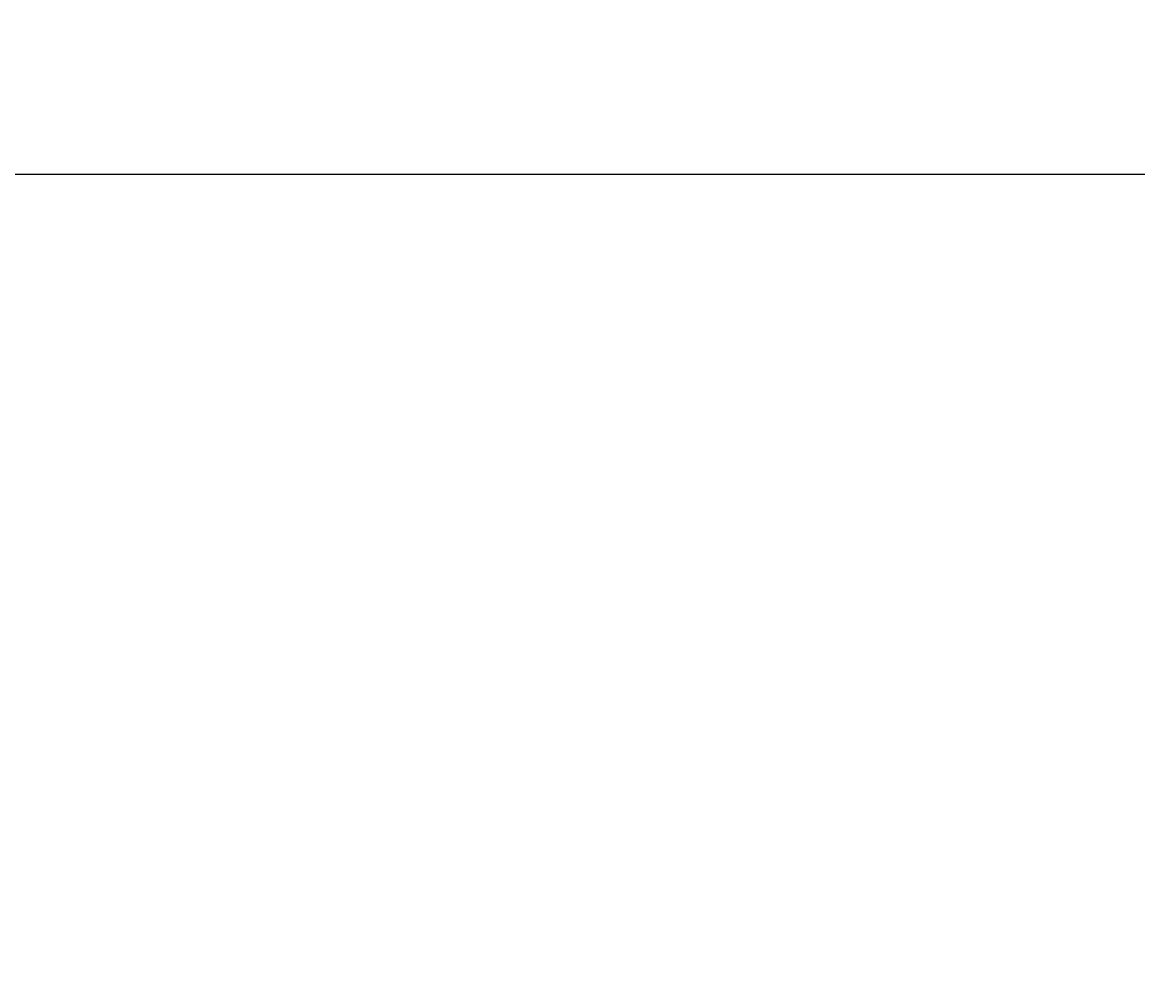
# Model space of a CAD drawing. Units: inches. Extents: x 35362 to 73946, y 43607 to 67532.
# Tile 106 of 134: x 50761 to 50905, y 48793 to 48917. Entities that reach past the tile are written whole.
import ezdxf

# ---------------------------------------------------------------- set-up
doc = ezdxf.new("R2010")
doc.units = ezdxf.units.IN
doc.header["$MEASUREMENT"] = 0
doc.layers.add('A-ANNO-DIMS', color=2, linetype='Continuous', lineweight=18)
doc.styles.get("Standard").update_dxf_attribs({"font": 'arial.ttf'})
doc.dimstyles.get("Standard").update_dxf_attribs({"dimtxt": 0.18, "dimasz": 0.18, "dimexe": 0.18, "dimexo": 0.0625, "dimgap": 0.09, "dimtad": 0, "dimtih": 1, "dimtoh": 1, "dimdec": 4, "dimzin": 0, "dimdsep": 46, "dimtxsty": 'Standard', "dimcen": 0.09, "dimadec": 0, "dimazin": 0, "dimtfac": 1, "dimtdec": 4, "dimtofl": 0, "dimtmove": 0, "dimatfit": 3, "dimfxl": 1, "dimtolj": 1, "dimtzin": 0, "dimarcsym": 0})

# ---------------------------------------------------------------- blocks, each defined once
blk = doc.blocks.new('*D11')
at = {"layer": 'A-ANNO-DIMS', "color": 0, "lineweight": -2, "transparency": 16777216}
for p, q in [((47978.66, 56028.77), (47978.66, 43606.68)), ((53109.76, 56028.77), (53109.76, 43606.68)), ((47978.84, 43606.86), (50543.87, 43606.86)), ((53109.58, 43606.86), (50544.55, 43606.86))]:
    blk.add_line(p, q, dxfattribs=at)
at = {"layer": 'A-ANNO-DIMS', "color": 0, "transparency": 16777216}
for points in [[(47978.84, 43606.89), (47978.84, 43606.83), (47978.66, 43606.86)], [(53109.58, 43606.89), (53109.58, 43606.83), (53109.76, 43606.86)]]:
    blk.add_solid(points, dxfattribs=at)
at = {"layer": 'Defpoints', "color": 0, "transparency": 16777216}
for p in [(47978.66, 56028.84), (53109.76, 56028.84), (53109.76, 43606.86)]:
    blk.add_point(p, dxfattribs=at)
at = {"layer": 'A-ANNO-DIMS', "color": 0, "transparency": 16777216, "insert": (50544.21, 43606.86), "char_height": 0.18, "attachment_point": 5}
blk.add_mtext('\\A1;5131', dxfattribs=at)
blk = doc.blocks.new('*D13')
at = {"layer": 'A-ANNO-DIMS', "color": 0, "lineweight": -2, "transparency": 16777216}
for p, q in [((48373.49, 51694.02), (48373.49, 43606.68)), ((51029.04, 51694.02), (51029.04, 43606.68)), ((48373.67, 43606.86), (49700.8, 43606.86)), ((51028.86, 43606.86), (49701.73, 43606.86))]:
    blk.add_line(p, q, dxfattribs=at)
at = {"layer": 'A-ANNO-DIMS', "color": 0, "transparency": 16777216}
for points in [[(48373.67, 43606.89), (48373.67, 43606.83), (48373.49, 43606.86)], [(51028.86, 43606.89), (51028.86, 43606.83), (51029.04, 43606.86)]]:
    blk.add_solid(points, dxfattribs=at)
at = {"layer": 'Defpoints', "color": 0, "transparency": 16777216}
for p in [(48373.49, 51694.09), (51029.04, 51694.09), (51029.04, 43606.86)]:
    blk.add_point(p, dxfattribs=at)
at = {"layer": 'A-ANNO-DIMS', "color": 0, "transparency": 16777216, "insert": (49701.27, 43606.86), "char_height": 0.18, "attachment_point": 5}
blk.add_mtext('\\A1;2655.6', dxfattribs=at)
blk = doc.blocks.new('*D17')
at = {"layer": 'A-ANNO-DIMS', "color": 0, "lineweight": -2, "transparency": 16777216}
for p, q in [((49923.31, 61293.22), (49923.31, 43606.68)), ((51913.93, 61293.22), (51913.93, 43606.68)), ((49923.49, 43606.86), (50918.16, 43606.86)), ((51913.75, 43606.86), (50919.07, 43606.86))]:
    blk.add_line(p, q, dxfattribs=at)
at = {"layer": 'A-ANNO-DIMS', "color": 0, "transparency": 16777216}
for points in [[(49923.49, 43606.89), (49923.49, 43606.83), (49923.31, 43606.86)], [(51913.75, 43606.89), (51913.75, 43606.83), (51913.93, 43606.86)]]:
    blk.add_solid(points, dxfattribs=at)
at = {"layer": 'Defpoints', "color": 0, "transparency": 16777216}
for p in [(49923.31, 61293.29), (51913.93, 61293.29), (51913.93, 43606.86)]:
    blk.add_point(p, dxfattribs=at)
at = {"layer": 'A-ANNO-DIMS', "color": 0, "transparency": 16777216, "insert": (50918.62, 43606.86), "char_height": 0.18, "attachment_point": 5}
blk.add_mtext('\\A1;1990.6', dxfattribs=at)
blk = doc.blocks.new('*D67')
at = {"layer": 'A-ANNO-DIMS', "color": 0, "lineweight": -2, "transparency": 16777216}
for p, q in [((56873.54, 53351.53), (35361.77, 53351.53)), ((35361.95, 53351.35), (35361.95, 49400.89)), ((35361.95, 45450.07), (35361.95, 49400.53)), ((53793.58, 45449.89), (35361.77, 45449.89))]:
    blk.add_line(p, q, dxfattribs=at)
at = {"layer": 'A-ANNO-DIMS', "color": 0, "transparency": 16777216}
for points in [[(35361.92, 53351.35), (35361.98, 53351.35), (35361.95, 53351.53)], [(35361.92, 45450.07), (35361.98, 45450.07), (35361.95, 45449.89)]]:
    blk.add_solid(points, dxfattribs=at)
at = {"layer": 'Defpoints', "color": 0, "transparency": 16777216}
for p in [(35361.95, 53351.53), (56873.6, 53351.53), (53793.64, 45449.89)]:
    blk.add_point(p, dxfattribs=at)
at = {"layer": 'A-ANNO-DIMS', "color": 0, "transparency": 16777216, "insert": (35361.95, 49400.71), "char_height": 0.18, "attachment_point": 5}
blk.add_mtext('\\A1;7901.6', dxfattribs=at)
blk = doc.blocks.new('*D89')
at = {"layer": 'A-ANNO-DIMS', "color": 0, "lineweight": -2, "transparency": 16777216}
for p, q in [((53707.72, 48897.74), (35361.77, 48897.74)), ((35361.95, 48897.56), (35361.95, 48303.16)), ((35361.95, 47708.4), (35361.95, 48302.8)), ((53707.72, 47708.22), (35361.77, 47708.22))]:
    blk.add_line(p, q, dxfattribs=at)
at = {"layer": 'A-ANNO-DIMS', "color": 0, "transparency": 16777216}
for points in [[(35361.92, 48897.56), (35361.98, 48897.56), (35361.95, 48897.74)], [(35361.92, 47708.4), (35361.98, 47708.4), (35361.95, 47708.22)]]:
    blk.add_solid(points, dxfattribs=at)
at = {"layer": 'Defpoints', "color": 0, "transparency": 16777216}
for p in [(53707.78, 48897.74), (35361.95, 47708.22), (53707.78, 47708.22)]:
    blk.add_point(p, dxfattribs=at)
at = {"layer": 'A-ANNO-DIMS', "color": 0, "transparency": 16777216, "insert": (35361.95, 48302.98), "char_height": 0.18, "attachment_point": 5}
blk.add_mtext('\\A1;1189.5', dxfattribs=at)
blk = doc.blocks.new('*D107')
at = {"layer": 'A-ANNO-DIMS', "color": 0, "lineweight": -2, "transparency": 16777216}
for p, q in [((50139.56, 59850.01), (50139.56, 43606.68)), ((51320.81, 59850.01), (51320.81, 43606.68)), ((50139.74, 43606.86), (50729.73, 43606.86)), ((51320.63, 43606.86), (50730.64, 43606.86))]:
    blk.add_line(p, q, dxfattribs=at)
at = {"layer": 'A-ANNO-DIMS', "color": 0, "transparency": 16777216}
for points in [[(50139.74, 43606.89), (50139.74, 43606.83), (50139.56, 43606.86)], [(51320.63, 43606.89), (51320.63, 43606.83), (51320.81, 43606.86)]]:
    blk.add_solid(points, dxfattribs=at)
at = {"layer": 'Defpoints', "color": 0, "transparency": 16777216}
for p in [(50139.56, 59850.08), (51320.81, 59850.08), (51320.81, 43606.86)]:
    blk.add_point(p, dxfattribs=at)
at = {"layer": 'A-ANNO-DIMS', "color": 0, "transparency": 16777216, "insert": (50730.19, 43606.86), "char_height": 0.18, "attachment_point": 5}
blk.add_mtext('\\A1;1181.3', dxfattribs=at)

msp = doc.modelspace()

# ---------------------------------------------------------------- dimensions: what is measured, and where the dimension line sits
at = {"layer": 'A-ANNO-DIMS'}
for base, p1, p2, override, picture, middle in [((51913.931, 43606.859), (49923.307, 61293.286), (51913.931, 61293.286), {"dimdec": 1, "dimlfac": 1, "dimrnd": 0, "dimzin": 0, "dimdsep": 46, "dimlunit": 2}, '*D17', (50918.619, 43606.859)), ((51320.8133, 43606.859), (50139.5627, 59850.0769), (51320.8133, 59850.0769), {"dimdec": 1, "dimlfac": 1, "dimrnd": 0, "dimzin": 0, "dimdsep": 46, "dimlunit": 2}, '*D107', (50730.188, 43606.859)), ((53109.76, 43606.859), (47978.665, 56028.836), (53109.76, 56028.836), {"dimdec": 0, "dimlfac": 1, "dimrnd": 0, "dimzin": 0, "dimdsep": 46, "dimlunit": 2}, '*D11', (50544.212, 43606.859)), ((51029.043, 43606.859), (48373.492, 51694.087), (51029.043, 51694.087), {"dimdec": 1, "dimlfac": 1, "dimrnd": 0, "dimzin": 0, "dimdsep": 46, "dimlunit": 2}, '*D13', (49701.267, 43606.859))]:
    dim = msp.add_linear_dim(base=base, p1=p1, p2=p2, dimstyle='Standard', override=override, dxfattribs=at)
    dim.commit()
    dim.dimension.update_dxf_attribs({"geometry": picture, "text_midpoint": middle})
for base, p1, p2, picture, middle in [((35361.949, 53351.529), (53793.638, 45449.894), (56873.602, 53351.529), '*D67', (35361.949, 49400.712)), ((35361.949, 47708.216), (53707.781, 48897.738), (53707.781, 47708.216), '*D89', (35361.949, 48302.977))]:
    dim = msp.add_linear_dim(base=base, p1=p1, p2=p2, angle=90, dimstyle='Standard', override={"dimdec": 1, "dimlfac": 1, "dimrnd": 0, "dimzin": 0, "dimdsep": 46, "dimlunit": 2}, dxfattribs=at)
    dim.commit()
    dim.dimension.update_dxf_attribs({"geometry": picture, "text_midpoint": middle})

doc.saveas('drawing.dxf')
